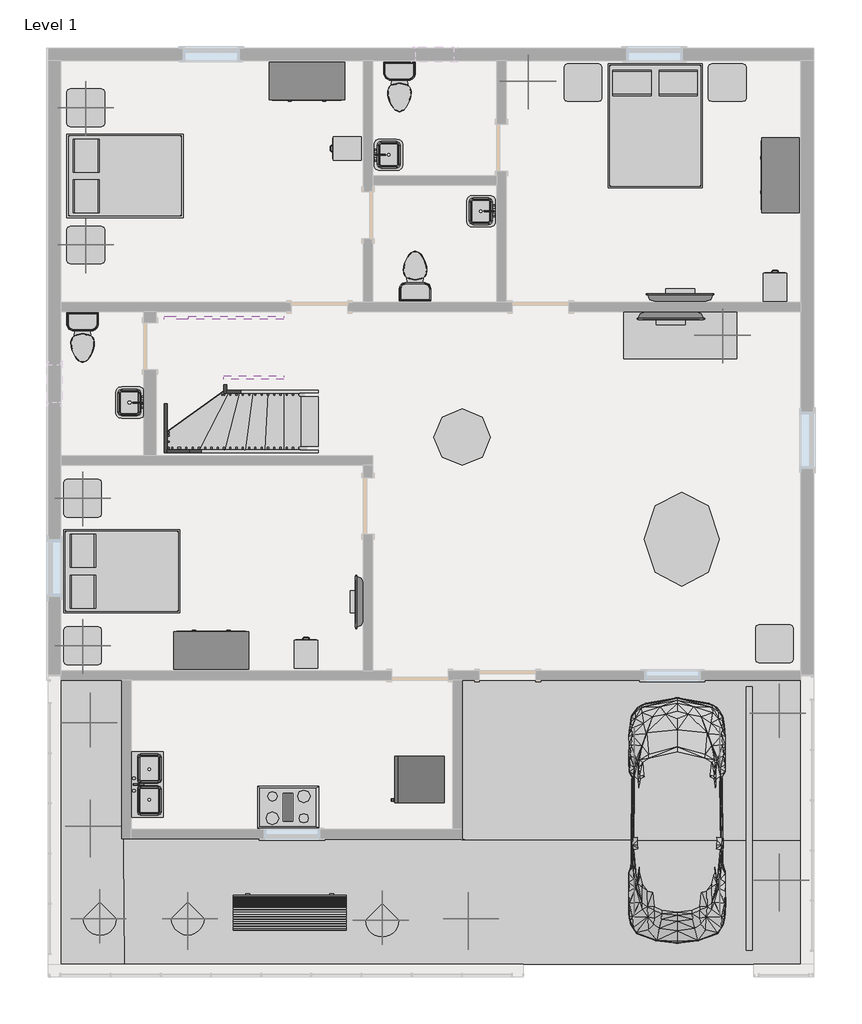
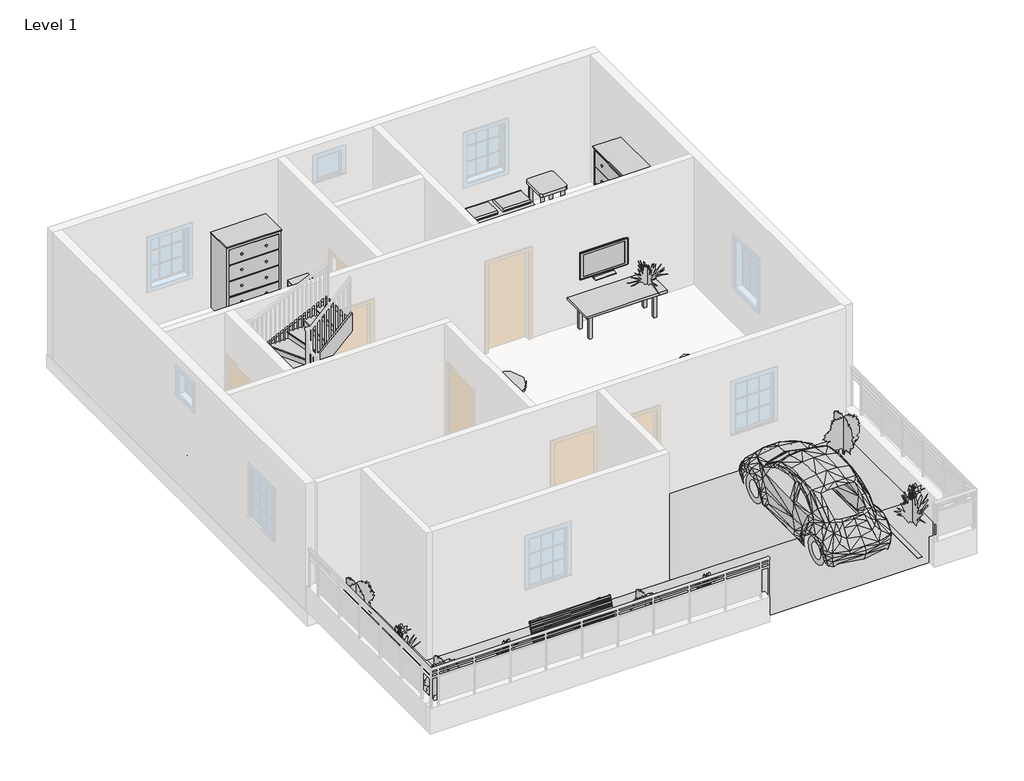
# One storey, part 3 of 3: 22 furniture elements, 15 geographic elements, 10 flow terminals, 8 members, 7 proxies, 1 stair flight.
"""IFC4 building model written with IfcOpenShell, lengths in millimetres."""

from ifc_helpers import new_model, si_unit, frame, origin, place, context, project, spatial, polyline, outline, extrude, triangles, transform, mapped, element, save
from components import proxy_bb1e6e30, parking_space_9_x_18_90_deg_fdd9e8f5, rpc_beetle_rpc_beetle_3ce7ba48, proxy_a13a33b2, flow_terminal_accce45a, flow_terminal_a53be723, flow_terminal_62a433f7, toilet_domestic_3d_toilet_domestic_3d_f7549cf7, toilet_domestic_3d_toilet_domestic_3d_183bbd19, furniture_c8abb964, furniture_1d2926bd, furniture_552c1472, furniture_9fa109b2, furniture_56245f3a, furniture_7a3aaa4f, furniture_905aceb5, furniture_743965d2, furniture_31d08a24, furniture_62ce4b1f, geographic_element_235d1464, rpc_plant_tropical_55f6ff97, rpc_plant_tropical_agave_1_5_93a2a214, rpc_plant_tropical_jungle_flame_3_9c4808c2, stair_flight_6de66a2c

model = new_model("IFC4")

# Units and contexts
model_context = context("Model", 3, world=origin())
ifc_project = project(units=[si_unit("LENGTHUNIT", "METRE", prefix="MILLI")], contexts=[model_context])

# Site, building, storey
site = spatial("IfcSite", under=ifc_project)
building = spatial("IfcBuilding", under=site)
storey = spatial("IfcBuildingStorey", under=building, Name="Level 1", Elevation=0.0)

# Proxies
placement = place(None, origin())
element("IfcBuildingElementProxy", 1, Name="Building Element Proxy", at=placement, inside=storey, context=model_context, shape_type="Tessellation", body=[
    triangles([(-13407.4397644, 1919.2116325, 0.0), (-12416.8397644, 1919.2116325, 0.0), (-13407.4397644, -2678.1882706, 0.0), (-12376.0190002, -2678.1882706, 0.0)], [[1, 3, 2], [4, 2, 3]], closed=False),
])
element("IfcBuildingElementProxy", 2, Name="Building Element Proxy", at=placement, inside=storey, context=model_context, shape_type="Tessellation", body=[
    triangles([(-12416.8397644, -646.188319, 0.0), (-12368.8403687, -2678.1882706, 0.0), (-1418.6402973, -679.6734118, 0.0), (-1418.6402973, -2678.1882706, 0.0)], [[1, 2, 3], [4, 3, 2]], closed=False),
])
element("IfcBuildingElementProxy", 3, Name="Building Element Proxy", at=placement, inside=storey, context=model_context, shape_type="Tessellation", body=[
    triangles([(-6905.040152, -646.188319, 0.0), (-1418.6402973, -347.7382948, 0.0), (-1418.6402973, 1919.2116325, 0.0), (-6905.040152, 1919.2116325, 0.0), (-1418.6402973, -674.1753462, 0.0), (-3670.4974686, -708.459082, 0.0), (-6733.3855133, -702.9520781, 0.0)], [[4, 1, 7], [4, 7, 6], [6, 5, 2], [2, 3, 6], [6, 3, 4]], closed=False),
])
proxy_shape = proxy_bb1e6e30(model_context)
element("IfcBuildingElementProxy", 4, Name="Cook Top-4 Unit : 36\" x 20\"", ObjectType="Cook Top-4 Unit : 36\" x 20\"", at=placement, inside=storey, context=model_context, shape_type="MappedRepresentation", body=[
    mapped(proxy_shape, transform((-9724.4402453, -138.1883114, 0.0), x_axis=(1.0, 0.0, 0.0), y_axis=(0.0, 1.0, 0.0), z_axis=(0.0, 0.0, 1.0))),
])
parking_space_9_x_18_90_deg_shape = parking_space_9_x_18_90_deg_fdd9e8f5(model_context)
element("IfcBuildingElementProxy", 5, Name="Parking Space : 9' x 18' - 90 deg", ObjectType="Parking Space : 9' x 18' - 90 deg", at=placement, inside=storey, context=model_context, shape_type="MappedRepresentation", body=[
    mapped(parking_space_9_x_18_90_deg_shape, transform((-2256.8402453, -2449.5883114, 0.0), x_axis=(-1.0, 0.0, 0.0), y_axis=(0.0, -1.0, 0.0), z_axis=(0.0, 0.0, 1.0))),
])
rpc_beetle_rpc_beetle_shape = rpc_beetle_rpc_beetle_3ce7ba48(model_context)
element("IfcBuildingElementProxy", 6, Name="RPC Beetle : RPC Beetle", ObjectType="RPC Beetle : RPC Beetle", at=placement, inside=storey, context=model_context, shape_type="MappedRepresentation", body=[
    mapped(rpc_beetle_rpc_beetle_shape, transform((-3425.2402453, -1585.9883114, 0.0), x_axis=(1.0, 0.0, 0.0), y_axis=(0.0, 1.0, 0.0), z_axis=(0.0, 0.0, 1.0))),
])
proxy_2_shape = proxy_a13a33b2(model_context)
element("IfcBuildingElementProxy", 7, Name="Refrigerator : 30\" x 32\" RH", ObjectType="Refrigerator : 30\" x 32\" RH", at=placement, inside=storey, context=model_context, shape_type="MappedRepresentation", body=[
    mapped(proxy_2_shape, transform((-7582.9027453, 311.4627171, 0.0), x_axis=(0.0, -1.0000000000000007, 0.0), y_axis=(1.0000000000000007, 0.0, 0.0), z_axis=(0.0, 0.0, 1.0))),
])

# Flow terminals
flow_terminal_shape = flow_terminal_accce45a(model_context)
element("IfcFlowTerminal", 8, ObjectType="Floor Drain - Round : 5\" Strainer - 2\" Drain", at=placement, inside=storey, context=model_context, shape_type="MappedRepresentation", body=[
    mapped(flow_terminal_shape, transform((-7006.6402453, 11825.2116886, 0.0), x_axis=(1.0, 0.0, 0.0), y_axis=(0.0, 1.0, 0.0), z_axis=(0.0, 0.0, 1.0))),
])
element("IfcFlowTerminal", 9, ObjectType="Floor Drain - Round : 5\" Strainer - 2\" Drain", at=placement, inside=storey, context=model_context, shape_type="MappedRepresentation", body=[
    mapped(flow_terminal_shape, transform((-6752.6402453, 8281.9116886, 0.0), x_axis=(1.0, 0.0, 0.0), y_axis=(0.0, 1.0, 0.0), z_axis=(0.0, 0.0, 1.0))),
])
element("IfcFlowTerminal", 10, ObjectType="Floor Drain - Round : 5\" Strainer - 2\" Drain", at=placement, inside=storey, context=model_context, shape_type="MappedRepresentation", body=[
    mapped(flow_terminal_shape, transform((-13255.0402453, 5830.8116886, 0.0), x_axis=(1.0, 0.0, 0.0), y_axis=(0.0, 1.0, 0.0), z_axis=(0.0, 0.0, 1.0))),
])
flow_terminal_2_shape = flow_terminal_a53be723(model_context)
element("IfcFlowTerminal", 11, ObjectType="Sink Kitchen-Double : 42\" x 21\"", at=placement, inside=storey, context=model_context, shape_type="MappedRepresentation", body=[
    mapped(flow_terminal_2_shape, transform((-12008.0948442, 214.4224481, 0.0), x_axis=(0.0, 1.0000000000000002, 0.0), y_axis=(-1.0000000000000002, 0.0, 0.0), z_axis=(0.0, 0.0, 1.0))),
])
flow_terminal_3_shape = flow_terminal_62a433f7(model_context)
element("IfcFlowTerminal", 12, ObjectType="Sink Vanity-Square : 20\" x 18\"", at=placement, inside=storey, context=model_context, shape_type="MappedRepresentation", body=[
    mapped(flow_terminal_3_shape, transform((-8147.2948442, 10412.5224481, 0.0), x_axis=(0.0, 1.0, 0.0), y_axis=(-1.0, 0.0, 0.0), z_axis=(0.0, 0.0, 1.0))),
])
element("IfcFlowTerminal", 13, ObjectType="Sink Vanity-Square : 20\" x 18\"", at=placement, inside=storey, context=model_context, shape_type="MappedRepresentation", body=[
    mapped(flow_terminal_3_shape, transform((-6551.7856464, 9529.5009292, 0.0), x_axis=(0.0, -1.0000000000000004, 0.0), y_axis=(1.0000000000000004, 0.0, 0.0), z_axis=(0.0, 0.0, 1.0))),
])
element("IfcFlowTerminal", 14, ObjectType="Sink Vanity-Square : 20\" x 18\"", at=placement, inside=storey, context=model_context, shape_type="MappedRepresentation", body=[
    mapped(flow_terminal_3_shape, transform((-12241.3856464, 6430.7009292, 0.0), x_axis=(0.0, -1.0000000000000004, 0.0), y_axis=(1.0000000000000004, 0.0, 0.0), z_axis=(0.0, 0.0, 1.0))),
])
toilet_domestic_3d_toilet_domestic_3d_shape = toilet_domestic_3d_toilet_domestic_3d_f7549cf7(model_context)
toilet_domestic_3d_toilet_domestic_3d_2_shape = toilet_domestic_3d_toilet_domestic_3d_183bbd19(model_context)
element("IfcFlowTerminal", 15, ObjectType="Toilet-Domestic-3D : Toilet-Domestic-3D", at=placement, inside=storey, context=model_context, shape_type="MappedRepresentation", body=[
    mapped(toilet_domestic_3d_toilet_domestic_3d_shape, transform((-7921.0402453, 11432.1156613, 0.0), x_axis=(1.0, 0.0, 0.0), y_axis=(0.0, 1.0, 0.0), z_axis=(0.0, 0.0, 1.0))),
    mapped(toilet_domestic_3d_toilet_domestic_3d_2_shape, transform((-7921.0402453, 11432.1156613, 0.0), x_axis=(1.0, 0.0, 0.0), y_axis=(0.0, 1.0, 0.0), z_axis=(0.0, 0.0, 1.0))),
])
element("IfcFlowTerminal", 16, ObjectType="Toilet-Domestic-3D : Toilet-Domestic-3D", at=placement, inside=storey, context=model_context, shape_type="MappedRepresentation", body=[
    mapped(toilet_domestic_3d_toilet_domestic_3d_shape, transform((-7667.0402453, 8560.707716, 0.0), x_axis=(-1.0000000000000004, 0.0, 0.0), y_axis=(0.0, -1.0000000000000004, 0.0), z_axis=(0.0, 0.0, 1.0))),
    mapped(toilet_domestic_3d_toilet_domestic_3d_2_shape, transform((-7667.0402453, 8560.707716, 0.0), x_axis=(-1.0000000000000004, 0.0, 0.0), y_axis=(0.0, -1.0000000000000004, 0.0), z_axis=(0.0, 0.0, 1.0))),
])
element("IfcFlowTerminal", 17, ObjectType="Toilet-Domestic-3D : Toilet-Domestic-3D", at=placement, inside=storey, context=model_context, shape_type="MappedRepresentation", body=[
    mapped(toilet_domestic_3d_toilet_domestic_3d_shape, transform((-13051.8402453, 7374.4656613, 0.0), x_axis=(1.0, 0.0, 0.0), y_axis=(0.0, 1.0, 0.0), z_axis=(0.0, 0.0, 1.0))),
    mapped(toilet_domestic_3d_toilet_domestic_3d_2_shape, transform((-13051.8402453, 7374.4656613, 0.0), x_axis=(1.0, 0.0, 0.0), y_axis=(0.0, 1.0, 0.0), z_axis=(0.0, 0.0, 1.0))),
])

# Furniture
furniture_shape = furniture_c8abb964(model_context)
element("IfcFurniture", 18, ObjectType="Bed-Box : Double 53\" x 74\"", at=placement, inside=storey, context=model_context, shape_type="MappedRepresentation", body=[
    mapped(furniture_shape, transform((-12600.4697535, 9746.1592296, 0.0), x_axis=(0.0, 1.0, 0.0), y_axis=(-1.0, 0.0, 0.0), z_axis=(0.0, 0.0, 1.0))),
])
element("IfcFurniture", 19, ObjectType="Bed-Box : Double 53\" x 74\"", at=placement, inside=storey, context=model_context, shape_type="MappedRepresentation", body=[
    mapped(furniture_shape, transform((-12651.2697535, 3345.3592296, 0.0), x_axis=(0.0, 1.0, 0.0), y_axis=(-1.0, 0.0, 0.0), z_axis=(0.0, 0.0, 1.0))),
])
furniture_2_shape = furniture_1d2926bd(model_context)
element("IfcFurniture", 20, ObjectType="Bed-Box : Queen 60\" x 79\"", at=placement, inside=storey, context=model_context, shape_type="MappedRepresentation", body=[
    mapped(furniture_2_shape, transform((-4119.9927043, 11132.5411968, 0.0), x_axis=(1.0, 0.0, 0.0), y_axis=(0.0, 1.0, 0.0), z_axis=(0.0, 0.0, 1.0))),
])
furniture_3_shape = furniture_552c1472(model_context)
element("IfcFurniture", 21, ObjectType="Cabinet-File 3 Drawer : 15\" x 18\"", at=placement, inside=storey, context=model_context, shape_type="MappedRepresentation", body=[
    mapped(furniture_3_shape, transform((-8623.4559452, 10401.9152416, 0.0), x_axis=(0.0, -1.0000000000000004, 0.0), y_axis=(1.0000000000000004, 0.0, 0.0), z_axis=(0.0, 0.0, 1.0))),
])
element("IfcFurniture", 22, ObjectType="Cabinet-File 3 Drawer : 15\" x 18\"", at=placement, inside=storey, context=model_context, shape_type="MappedRepresentation", body=[
    mapped(furniture_3_shape, transform((-1965.6366924, 8139.7773885, 0.0), x_axis=(-1.000000000000001, 0.0, 0.0), y_axis=(0.0, -1.000000000000001, 0.0), z_axis=(0.0, 0.0, 1.0))),
])
element("IfcFurniture", 23, ObjectType="Cabinet-File 3 Drawer : 15\" x 18\"", at=placement, inside=storey, context=model_context, shape_type="MappedRepresentation", body=[
    mapped(furniture_3_shape, transform((-9560.2366924, 2196.1773885, 0.0), x_axis=(-1.0000000000000004, 0.0, 0.0), y_axis=(0.0, -1.0000000000000004, 0.0), z_axis=(0.0, 0.0, 1.0))),
])
furniture_4_shape = furniture_9fa109b2(model_context)
element("IfcFurniture", 24, ObjectType="Dresser : 48\" x 72\" x 24\"", at=placement, inside=storey, context=model_context, shape_type="MappedRepresentation", body=[
    mapped(furniture_4_shape, transform((-9150.4469855, 11985.1746427, 0.0), x_axis=(1.0, 0.0, 0.0), y_axis=(0.0, 1.0, 0.0), z_axis=(0.0, 0.0, 1.0))),
])
element("IfcFurniture", 25, ObjectType="Dresser : 48\" x 72\" x 24\"", at=placement, inside=storey, context=model_context, shape_type="MappedRepresentation", body=[
    mapped(furniture_4_shape, transform((-1385.6772912, 9828.8184288, 0.0), x_axis=(0.0, -1.0000000000000004, 0.0), y_axis=(1.0000000000000004, 0.0, 0.0), z_axis=(0.0, 0.0, 1.0))),
])
element("IfcFurniture", 26, ObjectType="Dresser : 48\" x 72\" x 24\"", at=placement, inside=storey, context=model_context, shape_type="MappedRepresentation", body=[
    mapped(furniture_4_shape, transform((-11238.2335052, 2038.6487345, 0.0), x_axis=(-1.0000000000000004, 0.0, 0.0), y_axis=(0.0, -1.0000000000000004, 0.0), z_axis=(0.0, 0.0, 1.0))),
])
furniture_5_shape = furniture_56245f3a(model_context)
element("IfcFurniture", 27, ObjectType="TV - Flat Screen : 32\"", at=placement, inside=storey, context=model_context, shape_type="MappedRepresentation", body=[
    mapped(furniture_5_shape, transform((-8563.778869, 3185.2671745, 914.4), x_axis=(0.0, -1.0000000000000004, 0.0), y_axis=(1.0000000000000004, 0.0, 0.0), z_axis=(0.0, 0.0, 1.0))),
])
furniture_6_shape = furniture_7a3aaa4f(model_context)
element("IfcFurniture", 28, ObjectType="TV - Flat Screen : 42\"", at=placement, inside=storey, context=model_context, shape_type="MappedRepresentation", body=[
    mapped(furniture_6_shape, transform((-3378.3847595, 8110.7106448, 914.4), x_axis=(-1.0000000000000004, 0.0, 0.0), y_axis=(0.0, -1.0000000000000004, 0.0), z_axis=(0.0, 0.0, 1.0))),
])
element("IfcFurniture", 29, ObjectType="TV - Flat Screen : 42\"", at=placement, inside=storey, context=model_context, shape_type="MappedRepresentation", body=[
    mapped(furniture_6_shape, transform((-3522.8957312, 7829.673065, 1041.4), x_axis=(1.0, 0.0, 0.0), y_axis=(0.0, 1.0, 0.0), z_axis=(0.0, 0.0, 1.0))),
])
furniture_7_shape = furniture_905aceb5(model_context)
element("IfcFurniture", 30, ObjectType="Table-Dining Round w Chairs : 36\" Diameter", at=placement, inside=storey, context=model_context, shape_type="MappedRepresentation", body=[
    mapped(furniture_7_shape, transform((-7008.7222125, 6041.0903771, 0.0), x_axis=(1.0, 0.0, 0.0), y_axis=(0.0, 1.0, 0.0), z_axis=(0.0, 0.0, 1.0))),
])
furniture_8_shape = furniture_743965d2(model_context)
element("IfcFurniture", 31, ObjectType="Table-Ellipse : 60\" x 48\"", at=placement, inside=storey, context=model_context, shape_type="MappedRepresentation", body=[
    mapped(furniture_8_shape, transform((-3349.0402453, 4205.2116886, 0.0), x_axis=(0.0, 1.0, 0.0), y_axis=(-1.0, 0.0, 0.0), z_axis=(0.0, 0.0, 1.0))),
])
furniture_9_shape = furniture_31d08a24(model_context)
element("IfcFurniture", 32, ObjectType="Table-End : 24\" x 24\"", at=placement, inside=storey, context=model_context, shape_type="MappedRepresentation", body=[
    mapped(furniture_9_shape, transform((-13309.5738756, 8815.3116886, 0.0), x_axis=(1.0, 0.0, 0.0), y_axis=(0.0, 1.0, 0.0), z_axis=(0.0, 0.0, 1.0))),
])
element("IfcFurniture", 33, ObjectType="Table-End : 24\" x 24\"", at=placement, inside=storey, context=model_context, shape_type="MappedRepresentation", body=[
    mapped(furniture_9_shape, transform((-13309.5738756, 11037.8116886, 0.0), x_axis=(1.0, 0.0, 0.0), y_axis=(0.0, 1.0, 0.0), z_axis=(0.0, 0.0, 1.0))),
])
element("IfcFurniture", 34, ObjectType="Table-End : 24\" x 24\"", at=placement, inside=storey, context=model_context, shape_type="MappedRepresentation", body=[
    mapped(furniture_9_shape, transform((-2920.9738756, 11444.2116886, 0.0), x_axis=(1.0, 0.0, 0.0), y_axis=(0.0, 1.0, 0.0), z_axis=(0.0, 0.0, 1.0))),
])
element("IfcFurniture", 35, ObjectType="Table-End : 24\" x 24\"", at=placement, inside=storey, context=model_context, shape_type="MappedRepresentation", body=[
    mapped(furniture_9_shape, transform((-5257.7738756, 11444.2116886, 0.0), x_axis=(1.0, 0.0, 0.0), y_axis=(0.0, 1.0, 0.0), z_axis=(0.0, 0.0, 1.0))),
])
element("IfcFurniture", 36, ObjectType="Table-End : 24\" x 24\"", at=placement, inside=storey, context=model_context, shape_type="MappedRepresentation", body=[
    mapped(furniture_9_shape, transform((-2158.9738756, 2357.3616886, 0.0), x_axis=(1.0, 0.0, 0.0), y_axis=(0.0, 1.0, 0.0), z_axis=(0.0, 0.0, 1.0))),
])
element("IfcFurniture", 37, ObjectType="Table-End : 24\" x 24\"", at=placement, inside=storey, context=model_context, shape_type="MappedRepresentation", body=[
    mapped(furniture_9_shape, transform((-13360.3738756, 2325.6116886, 0.0), x_axis=(1.0, 0.0, 0.0), y_axis=(0.0, 1.0, 0.0), z_axis=(0.0, 0.0, 1.0))),
])
element("IfcFurniture", 38, ObjectType="Table-End : 24\" x 24\"", at=placement, inside=storey, context=model_context, shape_type="MappedRepresentation", body=[
    mapped(furniture_9_shape, transform((-13360.3738756, 4713.2116886, 0.0), x_axis=(1.0, 0.0, 0.0), y_axis=(0.0, 1.0, 0.0), z_axis=(0.0, 0.0, 1.0))),
])
furniture_10_shape = furniture_62ce4b1f(model_context)
element("IfcFurniture", 39, ObjectType="Table-Rectangular : 72\" x 30\"", at=placement, inside=storey, context=model_context, shape_type="MappedRepresentation", body=[
    mapped(furniture_10_shape, transform((-3374.4402453, 7507.2116886, 0.0), x_axis=(1.0, 0.0, 0.0), y_axis=(0.0, 1.0, 0.0), z_axis=(0.0, 0.0, 1.0))),
])

# Geographic elements
geographic_element_shape = geographic_element_235d1464(model_context)
element("IfcGeographicElement", 40, ObjectType="Park Bench : 72\"", at=placement, inside=storey, context=model_context, shape_type="MappedRepresentation", body=[
    mapped(geographic_element_shape, transform((-9699.0402453, -1814.5883114, 0.0), x_axis=(1.0, 0.0, 0.0), y_axis=(0.0, 1.0, 0.0), z_axis=(0.0, 0.0, 1.0))),
])
rpc_plant_tropical_shape = rpc_plant_tropical_55f6ff97(model_context)
element("IfcGeographicElement", 41, ObjectType="RPC Plant - Tropical", at=placement, inside=storey, context=model_context, shape_type="MappedRepresentation", body=[
    mapped(rpc_plant_tropical_shape, transform((-12924.8402453, -442.9883114, 0.0), x_axis=(1.0, 0.0, 0.0), y_axis=(0.0, 1.0, 0.0), z_axis=(0.0, 0.0, 1.0))),
])
element("IfcGeographicElement", 42, ObjectType="RPC Plant - Tropical", at=placement, inside=storey, context=model_context, shape_type="MappedRepresentation", body=[
    mapped(rpc_plant_tropical_shape, transform((-11350.0402453, -1941.5883114, 0.0), x_axis=(1.0, 0.0, 0.0), y_axis=(0.0, 1.0, 0.0), z_axis=(0.0, 0.0, 1.0))),
])
element("IfcGeographicElement", 43, ObjectType="RPC Plant - Tropical", at=placement, inside=storey, context=model_context, shape_type="MappedRepresentation", body=[
    mapped(rpc_plant_tropical_shape, transform((-6803.4402453, -1941.5883114, 0.0), x_axis=(1.0, 0.0, 0.0), y_axis=(0.0, 1.0, 0.0), z_axis=(0.0, 0.0, 1.0))),
])
element("IfcGeographicElement", 44, ObjectType="RPC Plant - Tropical", at=placement, inside=storey, context=model_context, shape_type="MappedRepresentation", body=[
    mapped(rpc_plant_tropical_shape, transform((-1774.2402453, -1319.2883114, 0.0), x_axis=(1.0, 0.0, 0.0), y_axis=(0.0, 1.0, 0.0), z_axis=(0.0, 0.0, 1.0))),
])
rpc_plant_tropical_agave_1_5_shape = rpc_plant_tropical_agave_1_5_93a2a214(model_context)
element("IfcGeographicElement", 45, ObjectType="RPC Plant - Tropical : Agave - 1.5'", at=placement, inside=storey, context=model_context, shape_type="MappedRepresentation", body=[
    mapped(rpc_plant_tropical_agave_1_5_shape, transform((-13001.0402453, 11190.2116886, 609.6), x_axis=(1.0, 0.0, 0.0), y_axis=(0.0, 1.0, 0.0), z_axis=(0.0, 0.0, 1.0))),
])
element("IfcGeographicElement", 46, ObjectType="RPC Plant - Tropical : Agave - 1.5'", at=placement, inside=storey, context=model_context, shape_type="MappedRepresentation", body=[
    mapped(rpc_plant_tropical_agave_1_5_shape, transform((-13001.0402453, 8967.7116886, 609.6), x_axis=(1.0, 0.0, 0.0), y_axis=(0.0, 1.0, 0.0), z_axis=(0.0, 0.0, 1.0))),
])
element("IfcGeographicElement", 47, ObjectType="RPC Plant - Tropical : Agave - 1.5'", at=placement, inside=storey, context=model_context, shape_type="MappedRepresentation", body=[
    mapped(rpc_plant_tropical_agave_1_5_shape, transform((-5838.2402453, 11622.0116886, 0.0), x_axis=(1.0, 0.0, 0.0), y_axis=(0.0, 1.0, 0.0), z_axis=(0.0, 0.0, 1.0))),
])
element("IfcGeographicElement", 48, ObjectType="RPC Plant - Tropical : Agave - 1.5'", at=placement, inside=storey, context=model_context, shape_type="MappedRepresentation", body=[
    mapped(rpc_plant_tropical_agave_1_5_shape, transform((-2688.6402453, 7507.2116886, 685.8), x_axis=(1.0, 0.0, 0.0), y_axis=(0.0, 1.0, 0.0), z_axis=(0.0, 0.0, 1.0))),
])
element("IfcGeographicElement", 49, ObjectType="RPC Plant - Tropical : Agave - 1.5'", at=placement, inside=storey, context=model_context, shape_type="MappedRepresentation", body=[
    mapped(rpc_plant_tropical_agave_1_5_shape, transform((-13051.8402453, 2478.0116886, 609.6), x_axis=(1.0, 0.0, 0.0), y_axis=(0.0, 1.0, 0.0), z_axis=(0.0, 0.0, 1.0))),
])
element("IfcGeographicElement", 50, ObjectType="RPC Plant - Tropical : Agave - 1.5'", at=placement, inside=storey, context=model_context, shape_type="MappedRepresentation", body=[
    mapped(rpc_plant_tropical_agave_1_5_shape, transform((-13051.8402453, 4865.6116886, 609.6), x_axis=(1.0, 0.0, 0.0), y_axis=(0.0, 1.0, 0.0), z_axis=(0.0, 0.0, 1.0))),
])
rpc_plant_tropical_jungle_flame_3_shape = rpc_plant_tropical_jungle_flame_3_9c4808c2(model_context)
element("IfcGeographicElement", 51, ObjectType="RPC Plant - Tropical : Jungle Flame - 3'", at=placement, inside=storey, context=model_context, shape_type="MappedRepresentation", body=[
    mapped(rpc_plant_tropical_jungle_flame_3_shape, transform((-12924.8402453, 1233.4116886, 0.0), x_axis=(1.0, 0.0, 0.0), y_axis=(0.0, 1.0, 0.0), z_axis=(0.0, 0.0, 1.0))),
])
element("IfcGeographicElement", 52, ObjectType="RPC Plant - Tropical : Jungle Flame - 3'", at=placement, inside=storey, context=model_context, shape_type="MappedRepresentation", body=[
    mapped(rpc_plant_tropical_jungle_flame_3_shape, transform((-12772.4402453, -1941.5883114, 0.0), x_axis=(1.0, 0.0, 0.0), y_axis=(0.0, 1.0, 0.0), z_axis=(0.0, 0.0, 1.0))),
])
element("IfcGeographicElement", 53, ObjectType="RPC Plant - Tropical : Jungle Flame - 3'", at=placement, inside=storey, context=model_context, shape_type="MappedRepresentation", body=[
    mapped(rpc_plant_tropical_jungle_flame_3_shape, transform((-1774.2402453, 1385.8116886, 0.0), x_axis=(1.0, 0.0, 0.0), y_axis=(0.0, 1.0, 0.0), z_axis=(0.0, 0.0, 1.0))),
])
element("IfcGeographicElement", 54, ObjectType="RPC Plant - Tropical : Jungle Flame - 3'", at=placement, inside=storey, context=model_context, shape_type="MappedRepresentation", body=[
    mapped(rpc_plant_tropical_jungle_flame_3_shape, transform((-8200.4402453, -1966.9883114, 0.0), x_axis=(1.0, 0.0, 0.0), y_axis=(0.0, 1.0, 0.0), z_axis=(0.0, 0.0, 1.0))),
])

# Members
element("IfcMember", 55, ObjectType="Stringer - 2\" Width", at=placement, inside=storey, context=model_context, shape_type="SweptSolid", body=[
    extrude(outline(polyline([(0.0, -9238.1085535), (229.639954, -9238.1085535), (1305.3956453, -11325.5257451), (962.500629, -11325.5257451), (0.0, -9457.870871), (0.0, -9238.1085535)])), frame((0.0, 5602.2116886, 0.0), z_axis=(0.0, 1.0, 0.0), x_axis=(0.0, 0.0, 1.0)), (0.0, 0.0, 1.0), 50.8),
])
element("IfcMember", 56, ObjectType="Stringer - 2\" Width", at=placement, inside=storey, context=model_context, shape_type="SweptSolid", body=[
    extrude(outline(polyline([(-11325.5257451, 5653.0116886), (-11325.5257451, 5602.2116886), (-11680.2402453, 5602.2116886), (-11680.2402453, 5653.0116886), (-11325.5257451, 5653.0116886)])), frame((0.0, 0.0, 962.500629), z_axis=(0.0, 0.0, 1.0), x_axis=(1.0, 0.0, 0.0)), (0.0, 0.0, 1.0), 342.8950162),
])
element("IfcMember", 57, ObjectType="Stringer - 2\" Width", at=placement, inside=storey, context=model_context, shape_type="SweptSolid", body=[
    extrude(outline(polyline([(5602.2116886, 1000.5956453), (5602.2116886, 1289.0952212), (7724.2315713, 1969.9972697), (7761.2116886, 1969.9972697), (7761.2116886, 1638.9682298), (5771.7341716, 1000.5956453), (5602.2116886, 1000.5956453)])), frame((-11731.0402453, 0.0, 0.0), z_axis=(1.0, 0.0, 0.0), x_axis=(0.0, 1.0, 0.0)), (0.0, 0.0, 1.0), 50.8),
])
element("IfcMember", 58, ObjectType="Stringer - 2\" Width", at=placement, inside=storey, context=model_context, shape_type="SweptSolid", body=[
    extrude(outline(polyline([(-11731.0402453, 7761.2116886), (-11731.0402453, 7812.0116886), (-11342.0021142, 7812.0116886), (-11342.0021142, 7761.2116886), (-11731.0402453, 7761.2116886)])), frame((0.0, 0.0, 1649.8904473), z_axis=(0.0, 0.0, 1.0), x_axis=(1.0, 0.0, 0.0)), (0.0, 0.0, 1.0), 320.1068224),
])
element("IfcMember", 59, ObjectType="Stringer - 2\" Width", at=placement, inside=storey, context=model_context, shape_type="SweptSolid", body=[
    extrude(outline(polyline([(1969.9972697, -11342.0021142), (1649.8904473, -11342.0021142), (2373.9158336, -9796.9085535), (2694.022656, -9796.9085535), (1969.9972697, -11342.0021142)])), frame((0.0, 7761.2116886, 0.0), z_axis=(0.0, 1.0, 0.0), x_axis=(0.0, 0.0, 1.0)), (0.0, 0.0, 1.0), 50.8),
])
element("IfcMember", 60, ObjectType="Stringer - 2\" Width", at=placement, inside=storey, context=model_context, shape_type="SweptSolid", body=[
    extrude(outline(polyline([(0.0, -9238.1085535), (176.1764461, -9238.1085535), (1380.418648, -10715.0402453), (987.1410923, -10715.0402453), (0.0, -9504.370198), (0.0, -9238.1085535)])), frame((0.0, 6567.4116886, 0.0), z_axis=(0.0, 1.0, 0.0), x_axis=(0.0, 0.0, 1.0)), (0.0, 0.0, 1.0), 50.8),
])
element("IfcMember", 61, ObjectType="Stringer - 2\" Width", at=placement, inside=storey, context=model_context, shape_type="SweptSolid", body=[
    extrude(outline(polyline([(6567.4116886, 1028.5617647), (6567.4116886, 1573.2682978), (6786.732174, 1947.8002622), (6796.0116886, 1947.8002622), (6796.0116886, 1360.465107), (6601.6539059, 1028.5617647), (6567.4116886, 1028.5617647)])), frame((-10765.8402453, 0.0, 0.0), z_axis=(1.0, 0.0, 0.0), x_axis=(0.0, 1.0, 0.0)), (0.0, 0.0, 1.0), 50.8),
])
element("IfcMember", 62, ObjectType="Stringer - 2\" Width", at=placement, inside=storey, context=model_context, shape_type="SweptSolid", body=[
    extrude(outline(polyline([(1947.8002622, -10765.8402453), (1519.8508308, -10765.8402453), (2474.7821756, -9796.9085535), (2902.731607, -9796.9085535), (1947.8002622, -10765.8402453)])), frame((0.0, 6796.0116886, 0.0), z_axis=(0.0, 1.0, 0.0), x_axis=(0.0, 0.0, 1.0)), (0.0, 0.0, 1.0), 50.8),
])

# Stair flight
stair_flight_shape = stair_flight_6de66a2c(model_context)
element("IfcStairFlight", 63, ObjectType="2\" Tread 1\" Nosing 1/4\" Riser", at=placement, inside=storey, context=model_context, shape_type="MappedRepresentation", body=[
    mapped(stair_flight_shape, transform((0.0, 0.0, 0.0), x_axis=(1.0, 0.0, 0.0), y_axis=(0.0, 1.0, 0.0), z_axis=(0.0, 0.0, 1.0))),
])

save(model, "model.ifc")

# Revit data of these elements
# Type "Cook Top-4 Unit : 36\" x 20\""
#   Assembly Code = "E1090400"
#   Depth = 2' - 0"
#   Width = 3' - 0"
#   Burner Material = Steel, Chrome Plated
#   Cooktop Material = Steel, Polished
#   Default Elevation = 0
# Type "Parking Space : 9' x 18' - 90 deg"
#   Angle = 90.00°
#   Parking Length = 18' - 0"
#   Parking Width = 9' - 0"
#   pl = 14' - 0"
#   pw = 8' - 0"
# Type "RPC Beetle : RPC Beetle"
#   built-in parameter 1005195 = "RPC-16-0U6E-L4EG-ENH1-J3KF-SVEL-0TX4-C0"
#   Height = 0
# Type "Refrigerator : 30\" x 32\" RH"
#   Label = "REF."
#   Assembly Code = "E1090400"
#   Depth = 2' - 7 3/4"
#   Handle = 2' - 3"
#   Height = 5' - 10"
#   Rear Clearance = 0' - 2"
#   Top Door Height = 1' - 8"
#   Width = 2' - 5 3/8"
#   Material = Steel, Paint Finish, Ivory, Glossy
#   Default Elevation = 0
# Type "Floor Drain - Round : 5\" Strainer - 2\" Drain"
#   WFU = 2
#   Strainer Height = 0' - 3 1/4"
#   Strainer Radius = 0' - 2 1/2"
#   Strainer Diameter = 0' - 5"
#   Radius 6 = 0' - 0 5/8"
#   Radius 5 = 0' - 1 1/4"
#   Radius 4 = 0' - 1 7/8"
#   Radius 2 = 0' - 3.04167"
#   Radius 1 = 0' - 2.02083"
#   Radius 3 = 0' - 2 1/32"
#   Pipe Radius = 1"
#   Pipe Diameter = 2"
#   Height 2 = 0' - 0.725"
#   Height 1 = 0' - 1 13/16"
#   Body Radius = 0' - 4 1/16"
#   Body Height = 0' - 3 5/8"
#   Body Diameter = 0' - 8 1/8"
#   Drain Material = none
#   HWFU = 0
#   Default Elevation = 0
#   CWFU = 0
# Type "Sink Kitchen-Double : 42\" x 21\""
#   Assembly Code = "D2010410"
#   Counter Height = 3' - 0"
#   Depth = 1' - 9"
#   Width = 3' - 6"
#   Faucet Material = Steel, Polished
#   Sink Material = Steel, Polished
#   Default Elevation = 0
# Type "Sink Vanity-Square : 20\" x 18\""
#   Assembly Code = "D2010400"
#   Counter Height = 2' - 7"
#   Depth = 1' - 6"
#   Width = 1' - 8"
#   Basin Material = Porcelain, Linen
#   Faucet Material = Steel, Polished
#   Default Elevation = 0
# Type "Toilet-Domestic-3D : Toilet-Domestic-3D"
#   Assembly Code = "D2010110"
#   Toilet - Bowl/Basin Material = Porcelain, Linen
#   Toilet - Seat Material = Laminate, Linen, Matte
#   Default Elevation = 0
# Type "Bed-Box : Double 53\" x 74\""
#   Assembly Code = "E2020200"
#   Length = 6' - 2"
#   Width = 4' - 5"
#   Frame Material = Birch
#   Mattress Material = Linen, White
#   Default Elevation = 0
# Type "Bed-Box : Queen 60\" x 79\""
#   Assembly Code = "E2020200"
#   Length = 6' - 7"
#   Width = 5' - 0"
#   Frame Material = Birch
#   Mattress Material = Linen, White
#   Default Elevation = 0
# Type "Cabinet-File 3 Drawer : 15\" x 18\""
#   Assembly Code = "E2020200"
#   Depth = 1' - 6"
#   Height = 3' - 5"
#   Width = 1' - 3"
#   Cabinet Material = Steel, Paint Finish, Ivory, Glossy
#   Handle Material = Steel, Chrome Plated
#   Default Elevation = 0
# Type "Dresser : 48\" x 72\" x 24\""
#   Assembly Code = "E2020200"
#   Depth = 2' - 0"
#   Height = 6' - 0"
#   Width = 4' - 0"
#   Dresser Material = Laminate - Ivory, Glossy
#   Drawer Material = Laminate, Ivory, Matte
#   Knob Material = Cherry
#   Default Elevation = 0
# Type "TV - Flat Screen : 32\""
#   SinAng = 0' - 0.0193"
#   L = 2' - 3.79372"
#   H = 1' - 3.6354"
#   Thickness = 0' - 4.33071"
#   Diagonal = 2' - 7.88976"
#   CosAng = 0' - 0.03431"
#   Stand [instance default] = yes
#   Default Elevation = 0
# Type "TV - Flat Screen : 42\""
#   SinAng = 0' - 0.0193"
#   L = 3' - 0.71517"
#   H = 1' - 8.65418"
#   Thickness = 0' - 4.33071"
#   Diagonal = 3' - 6.12598"
#   CosAng = 0' - 0.03431"
#   Stand [instance default] = yes
#   Default Elevation = 0
# Type "Table-Dining Round w Chairs : 36\" Diameter"
#   Assembly Code = "E2020200"
#   Radius = 1' - 6"
#   Diameter = 3' - 0"
#   Height = 2' - 6"
#   Chairs = 4
#   Base Material = Pine
#   Top Material = Laminate, Linen, Matte
#   Default Elevation = 0
# Type "Table-Ellipse : 60\" x 48\""
#   Assembly Code = "E2020200"
#   Half Width = 2' - 0"
#   Half Length = 2' - 6"
#   Height = 2' - 6"
#   Length = 5' - 0"
#   Width = 4' - 0"
#   Base Material = Birch
#   Top Material = Birch
#   Default Elevation = 0
# Type "Table-End : 24\" x 24\""
#   Assembly Code = "E2020200"
#   Height = 2' - 0"
#   Length = 2' - 0"
#   Width = 2' - 0"
#   Base Material = Birch
#   Top Material = Laminate, Ivory, Matte
#   Default Elevation = 0
# Type "Table-Rectangular : 72\" x 30\""
#   Assembly Code = "E2020200"
#   Height = 2' - 3"
#   Length = 6' - 0"
#   Width = 2' - 6"
#   Base Material = Birch
#   Top Material = Birch
#   Default Elevation = 0
# Type "Park Bench : 72\""
#   Length = 6' - 0"
#   Seat Material = Wood - Teak
#   Frame Material = Steel, Paint Finish, Dark Gray, Matte
# Type "RPC Plant - Tropical"
#   built-in parameter 1005198 = "{2, 15},{39, RPC-16-FWM5-GM7X-C67P-4000-ST1L-LVER-AU},{1, 0},{1, 0},{2, 13},{1, 8},{5, Color},{1, 0},{1, 0},{3, 0.8},{3, 0.8},{3, 0.8},{1, 8},{7, BBoxMin},{1, 0},{1, 0},{1, 0},{1, 0},{1, 0},{1, 8},{7, BBoxMax},{1, 0},{1, 0},{1, 0},{1, 0},{1, 0},{2, 11},{9, RPCTypeId},{1, 0},{1, 0},{39, RPC-16-FWM5-GM7X-C67P-4000-ST1L-LVER-AU},{1, 6},{14, RPCPlantHeight},{1, 0},{1, 0},{1, 3},{2, 11},{7, keyword},{1, 0},{1, 0},{35, :RPCs:Shrubs [General]:Geometry:RPC},{2, 11},{8, category},{1, 0},{1, 0},{16, Shrubs [General]},{2, 11},{12, LocalizedUID},{1, 0},{1, 0},{10, Crane Lily},{2, 14},{6, Height},{1, 0},{1, 0},{1, 3},{1, 2},{16, Cast Reflections},{1, 0},{1, 0},{1, 0},{1, 2},{12, Cast Shadows},{1, 0},{1, 0},{1, 1},{1, 2},{9, Lock View},{1, 0},{1, 0},{1, 0},{1, 4},{5, ViewC},{1, 0},{1, 0},{1, 0},{21, assetlibrary_base.fbx},{1, 5},"
#   built-in parameter 1005195 = "RPC-16-FWM5-GM7X-C67P-4000-ST1L-LVER-AU"
#   Assembly Code = "G2050500"
#   Height = 3' - 0"
#   Default Elevation = 0
# Type "RPC Plant - Tropical : Agave - 1.5'"
#   built-in parameter 1005198 = "{2, 15},{39, RPC-16-G1GJ-63FX-7K5P-N000-ST1L-LVER-AU},{1, 0},{1, 0},{2, 13},{1, 8},{5, Color},{1, 0},{1, 0},{3, 0.8},{3, 0.8},{3, 0.8},{1, 8},{7, BBoxMin},{1, 0},{1, 0},{1, 0},{1, 0},{1, 0},{1, 8},{7, BBoxMax},{1, 0},{1, 0},{1, 0},{1, 0},{1, 0},{2, 11},{9, RPCTypeId},{1, 0},{1, 0},{39, RPC-16-G1GJ-63FX-7K5P-N000-ST1L-LVER-AU},{1, 6},{14, RPCPlantHeight},{1, 0},{1, 0},{3, 1.5},{2, 11},{7, keyword},{1, 0},{1, 0},{35, :RPCs:Plants [General]:Geometry:RPC},{2, 11},{8, category},{1, 0},{1, 0},{16, Plants [General]},{2, 11},{12, LocalizedUID},{1, 0},{1, 0},{5, Agave},{2, 14},{6, Height},{1, 0},{1, 0},{3, 1.5},{1, 2},{16, Cast Reflections},{1, 0},{1, 0},{1, 0},{1, 2},{12, Cast Shadows},{1, 0},{1, 0},{1, 1},{1, 2},{9, Lock View},{1, 0},{1, 0},{1, 0},{1, 4},{5, ViewC},{1, 0},{1, 0},{1, 0},{21, assetlibrary_base.fbx},{1, 5},"
#   built-in parameter 1005195 = "RPC-16-G1GJ-63FX-7K5P-N000-ST1L-LVER-AU"
#   Type Comments = "Agave"
#   Assembly Code = "G2050500"
#   Height = 1' - 6"
#   Default Elevation = 0
# Type "RPC Plant - Tropical : Jungle Flame - 3'"
#   built-in parameter 1005198 = "{2, 15},{39, RPC-16-FUVJ-JWG0-MWGK-8000-ST1L-LVER-AU},{1, 0},{1, 0},{2, 13},{1, 8},{5, Color},{1, 0},{1, 0},{3, 0.8},{3, 0.8},{3, 0.8},{1, 8},{7, BBoxMin},{1, 0},{1, 0},{1, 0},{1, 0},{1, 0},{1, 8},{7, BBoxMax},{1, 0},{1, 0},{1, 0},{1, 0},{1, 0},{2, 11},{9, RPCTypeId},{1, 0},{1, 0},{39, RPC-16-FUVJ-JWG0-MWGK-8000-ST1L-LVER-AU},{1, 6},{14, RPCPlantHeight},{1, 0},{1, 0},{1, 3},{2, 11},{7, keyword},{1, 0},{1, 0},{35, :RPCs:Shrubs [General]:Geometry:RPC},{2, 11},{8, category},{1, 0},{1, 0},{16, Shrubs [General]},{2, 11},{12, LocalizedUID},{1, 0},{1, 0},{12, Jungle Flame},{2, 14},{6, Height},{1, 0},{1, 0},{1, 3},{1, 2},{16, Cast Reflections},{1, 0},{1, 0},{1, 0},{1, 2},{12, Cast Shadows},{1, 0},{1, 0},{1, 1},{1, 2},{9, Lock View},{1, 0},{1, 0},{1, 0},{1, 4},{5, ViewC},{1, 0},{1, 0},{1, 0},{21, assetlibrary_base.fbx},{1, 5},"
#   built-in parameter 1005195 = "RPC-16-FUVJ-JWG0-MWGK-8000-ST1L-LVER-AU"
#   Type Comments = "Jungle Flame"
#   Assembly Code = "G2050500"
#   Height = 3' - 0"
#   Default Elevation = 0
# Elements 1, 2, 3 (IfcBuildingElementProxy)
#   Material = none
#   Phase Created = New Construction
# Element 4 (IfcBuildingElementProxy, "Cook Top-4 Unit : 36\" x 20\"")
#   Phase Created = New Construction
#   Materials on its faces: "Steel, Chrome Plated", "Steel, Polished"
# Element 5 (IfcBuildingElementProxy, "Parking Space : 9' x 18' - 90 deg")
#   Phase Created = New Construction
#   Materials on its faces: "Parking Stripe"
# Element 6 (IfcBuildingElementProxy, "RPC Beetle : RPC Beetle")
#   Phase Created = New Construction
# Element 7 (IfcBuildingElementProxy, "Refrigerator : 30\" x 32\" RH")
#   Phase Created = New Construction
#   Materials on its faces: "Steel, Paint Finish, Ivory, Glossy", "Steel, Chrome Plated"
# Element 8 (IfcFlowTerminal, "Floor Drain - Round : 5\" Strainer - 2\" Drain")
#   Mark = "3"
#   Phase Created = New Construction
# Element 9 (IfcFlowTerminal, "Floor Drain - Round : 5\" Strainer - 2\" Drain")
#   Mark = "4"
#   Phase Created = New Construction
# Element 10 (IfcFlowTerminal, "Floor Drain - Round : 5\" Strainer - 2\" Drain")
#   Mark = "10"
#   Phase Created = New Construction
# Element 11 (IfcFlowTerminal, "Sink Kitchen-Double : 42\" x 21\"")
#   Mark = "11"
#   Phase Created = New Construction
#   Materials on its faces: "Steel, Polished"
# Element 12 (IfcFlowTerminal, "Sink Vanity-Square : 20\" x 18\"")
#   Mark = "2"
#   Phase Created = New Construction
#   Materials on its faces: "Porcelain, Linen", "Steel, Polished"
# Element 13 (IfcFlowTerminal, "Sink Vanity-Square : 20\" x 18\"")
#   Mark = "6"
#   Phase Created = New Construction
#   Materials on its faces: "Porcelain, Linen", "Steel, Polished"
# Element 14 (IfcFlowTerminal, "Sink Vanity-Square : 20\" x 18\"")
#   Mark = "9"
#   Phase Created = New Construction
#   Materials on its faces: "Porcelain, Linen", "Steel, Polished"
# Element 15 (IfcFlowTerminal, "Toilet-Domestic-3D : Toilet-Domestic-3D")
#   Mark = "1"
#   Phase Created = New Construction
#   Materials on its faces: "Porcelain, Linen", "Laminate, Linen, Matte"
# Element 16 (IfcFlowTerminal, "Toilet-Domestic-3D : Toilet-Domestic-3D")
#   Mark = "5"
#   Phase Created = New Construction
#   Materials on its faces: "Porcelain, Linen", "Laminate, Linen, Matte"
# Element 17 (IfcFlowTerminal, "Toilet-Domestic-3D : Toilet-Domestic-3D")
#   Mark = "8"
#   Phase Created = New Construction
#   Materials on its faces: "Porcelain, Linen", "Laminate, Linen, Matte"
# Elements 18, 19 (IfcFurniture, "Bed-Box : Double 53\" x 74\"")
#   Phase Created = New Construction
#   Materials on its faces: "Birch", "Linen, White"
# Element 20 (IfcFurniture, "Bed-Box : Queen 60\" x 79\"")
#   Phase Created = New Construction
#   Materials on its faces: "Birch", "Linen, White"
# Elements 21, 22, 23 (IfcFurniture, "Cabinet-File 3 Drawer : 15\" x 18\"")
#   Phase Created = New Construction
#   Materials on its faces: "Steel, Chrome Plated", "Steel, Paint Finish, Ivory, Glossy"
# Elements 24, 25, 26 (IfcFurniture, "Dresser : 48\" x 72\" x 24\"")
#   Phase Created = New Construction
#   Materials on its faces: "Laminate, Ivory, Matte", "Cherry", "Laminate - Ivory, Glossy"
# Element 27 (IfcFurniture, "TV - Flat Screen : 32\"")
#   Stand = yes
#   Phase Created = New Construction
#   Materials on its faces: "TV - Black", "TV - Glass", "TV - Screen"
# Elements 28, 29 (IfcFurniture, "TV - Flat Screen : 42\"")
#   Stand = yes
#   Phase Created = New Construction
#   Materials on its faces: "TV - Black", "TV - Glass", "TV - Screen"
# Element 30 (IfcFurniture, "Table-Dining Round w Chairs : 36\" Diameter")
#   Phase Created = New Construction
#   Materials on its faces: "Pine", "Laminate, Linen, Matte"
# Element 31 (IfcFurniture, "Table-Ellipse : 60\" x 48\"")
#   Phase Created = New Construction
#   Materials on its faces: "Birch"
# Elements 32, 33, 34, 35, 36, 37, 38 (IfcFurniture, "Table-End : 24\" x 24\"")
#   Phase Created = New Construction
#   Materials on its faces: "Laminate, Ivory, Matte", "Birch"
# Element 39 (IfcFurniture, "Table-Rectangular : 72\" x 30\"")
#   Phase Created = New Construction
#   Materials on its faces: "Birch"
# Element 40 (IfcGeographicElement, "Park Bench : 72\"")
#   Phase Created = New Construction
#   Materials on its faces: "Wood - Teak", "Steel, Paint Finish, Dark Gray, Matte"
# Elements 41, 42, 43, 44 (IfcGeographicElement, "RPC Plant - Tropical")
#   Phase Created = New Construction
# Elements 45, 46, 47, 48, 49, 50 (IfcGeographicElement, "RPC Plant - Tropical : Agave - 1.5'")
#   Phase Created = New Construction
# Elements 51, 52, 53, 54 (IfcGeographicElement, "RPC Plant - Tropical : Jungle Flame - 3'")
#   Phase Created = New Construction
# Elements 55, 56, 57, 58, 59, 60, 61, 62 (IfcMember, "Stringer - 2\" Width")
#   Phase Created = New Construction
# Element 63 (IfcStairFlight, "2\" Tread 1\" Nosing 1/4\" Riser")
#   Phase Created = New Construction
# Materials
#   "Steel, Chrome Plated": class "Metal", colour RGB 17 17 17, transparency 0, Description = "Chromiuim plated steel", Cost = 0
#   "Steel, Polished": class "Metal", colour RGB 57 57 57, transparency 0, Description = "Polished steel", Cost = 0
#   "Steel, Paint Finish, Ivory, Glossy": class "Metal", colour RGB 247 247 239, transparency 0, Description = "Steel, paint finish, ivory, glossy", Cost = 0
#   "Porcelain, Linen": class "Ceramic", colour RGB 249 239 230, transparency 0, Description = "Porcelain, linen", Cost = 0
#   "Laminate, Linen, Matte": class "Plastic", colour RGB 249 239 230, transparency 0, Description = "Plastic Laminate - Linen, Matte", Cost = 0
#   "Birch": class "Wood", colour RGB 224 178 126, transparency 0, Description = "Betula Alleghaniensis", Cost = 0
#   "Linen, White": class "Textile", colour RGB 247 247 239, transparency 0, Description = "Linen, white", Cost = 0
#   "Laminate - Ivory, Glossy": colour RGB 247 247 239, transparency 0
#   "Laminate, Ivory, Matte": class "Plastic", colour RGB 247 247 239, transparency 0, Description = "Plastic Laminate - Ivory, Matte", Cost = 0
#   "Cherry": class "Wood", colour RGB 226 177 128, transparency 0, Description = "Prunus Serotina", Cost = 0
#   "Pine": class "Wood", colour RGB 223 192 134, transparency 0, Description = "Pinus Echinata", Cost = 0
#   "Wood - Teak": class "Wood", colour RGB 120 73 19, transparency 0
#   "Steel, Paint Finish, Dark Gray, Matte": class "Metal", colour RGB 98 98 98, transparency 0, Description = "Steel, paint finish, dark gray, matte", Cost = 0
#   "Parking Stripe": class "Paint", colour RGB 250 250 91, transparency 0
#   "TV - Black": colour RGB 49 49 49, transparency 0
#   "TV - Glass": colour RGB 157 157 157, transparency 0.9
#   "TV - Screen": colour RGB 0 0 0, transparency 0
